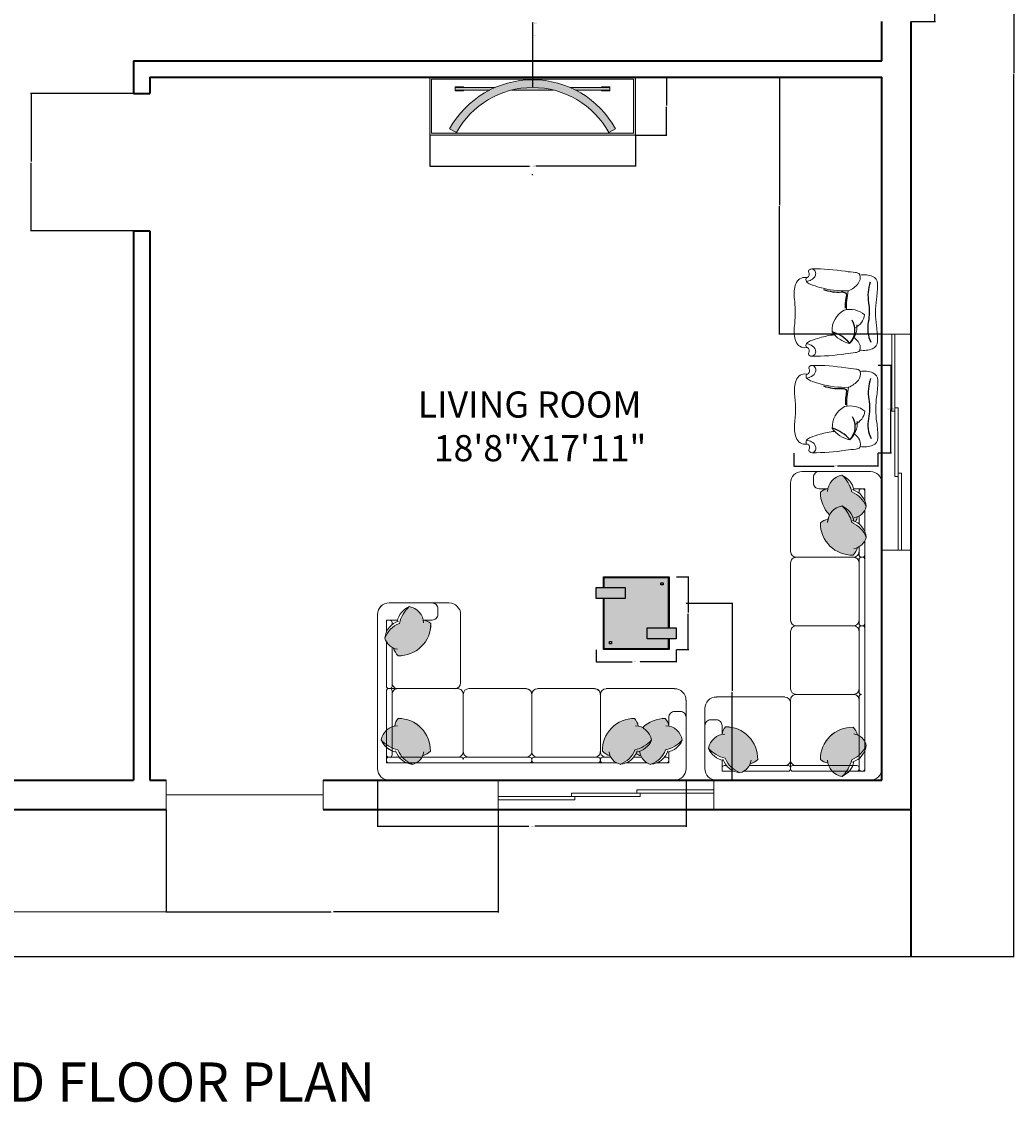
# Model space of a CAD drawing. Units: inches. Extents: x 1569 to 2779, y 1228 to 1844.
# Tile 2 of 6: x 1869 to 2173, y 1228 to 1559. Entities that reach past the tile are written whole.
import ezdxf

# ---------------------------------------------------------------- set-up
doc = ezdxf.new("R2010")
doc.units = ezdxf.units.IN
for name, color, linetype, lineweight in [('A-ANNO-DIMS', 2, 'Continuous', 18), ('A-ANNO-TEXT', 7, 'Continuous', 25), ('A-AREA-IDEN', 7, 'Continuous', 18), ('A-DOOR', 3, 'Continuous', 20), ('A-FLOR-EDGE', 7, 'Continuous', 25), ('A-FURN', 8, 'Continuous', 13), ('A-GLAZ', 5, 'Continuous', 18), ('A-WALL', 7, 'Continuous', 35), ('aparador', 36, 'Continuous', 9), ('moveis', 254, 'Continuous', 5)]:
    doc.layers.add(name, color=color, linetype=linetype, lineweight=lineweight)
doc.layers.add('IFF-FURN-DETAIL', color=250, linetype='Continuous')
doc.layers.add('MOBIL', color=7, linetype='Continuous')
doc.styles.get("Standard").update_dxf_attribs({"font": 'arial.ttf'})
doc.dimstyles.get("Standard").update_dxf_attribs({"dimtxt": 0.18, "dimasz": 0.18, "dimexe": 0.18, "dimexo": 0.0625, "dimgap": 0.09, "dimtad": 0, "dimtih": 1, "dimtoh": 1, "dimdec": 4, "dimzin": 0, "dimdsep": 46, "dimtxsty": 'Standard', "dimcen": 0.09, "dimadec": 0, "dimazin": 0, "dimtfac": 1, "dimtdec": 4, "dimtofl": 0, "dimtmove": 0, "dimatfit": 3, "dimfxl": 1, "dimtolj": 1, "dimtzin": 0, "dimarcsym": 0})

# ---------------------------------------------------------------- blocks, each defined once
blk = doc.blocks.new('Aparador ORGANICA Formatto')
at = {"layer": 'aparador', "ltscale": 0.3}
h = blk.add_hatch(color=256, dxfattribs=at)
h.dxf.hatch_style = 1
h.set_gradient(color1=(118, 213, 123), color2=(52, 168, 57), one_color=1, tint=0.43, name='INVCURVED')
h.paths.add_polyline_path([(0.8, 0.45), (-0.8, 0.45), (-0.8, 0), (0.8, 0)])
h.paths.add_polyline_path([(0.785, 0.435), (0.785, 0.015), (-0.785, 0.015), (-0.785, 0.435)], flags=16)
h.paths.add_polyline_path([(0.2911, 0.3699), (0.5365, 0.3699), (0.5365, 0.3757), (0.6011, 0.3757), (0.6011, 0.3699), (0.6011, 0.3499), (0.6011, 0.3441), (0.5365, 0.3441), (0.5365, 0.3499), (0.3338, 0.3499, -0.150336), (0.6449, 0.0488), (0.5923, 0.0199, 0.208852), (0.1632, 0.3499), (-0.1632, 0.3499, 0.208852), (-0.5923, 0.0199), (-0.6449, 0.0488, -0.150336), (-0.3338, 0.3499), (-0.5365, 0.3499), (-0.5365, 0.3441), (-0.6011, 0.3441), (-0.6011, 0.3499), (-0.6011, 0.3699), (-0.6011, 0.3757), (-0.5365, 0.3757), (-0.5365, 0.3699), (-0.2911, 0.3699, -0.206106)], flags=0)
h = blk.add_hatch(color=256, dxfattribs=at)
h.dxf.hatch_style = 1
h.set_gradient(color1=(135, 92, 69), color2=(0, 0, 0), one_color=1, name='INVCURVED')
h.paths.add_polyline_path([(-0.6449, 0.0488), (-0.5923, 0.0199, -0.590888), (0.5923, 0.0199), (0.6449, 0.0488, 0.590888)])
h = blk.add_hatch(color=256, dxfattribs=at)
h.dxf.hatch_style = 1
h.set_gradient(color1=(178, 189, 189), one_color=1, tint=1, name='CYLINDER')
h.paths.add_polyline_path([(-0.5365, 0.3757), (-0.6011, 0.3757), (-0.6011, 0.3699), (-0.5365, 0.3699)])
h.paths.add_polyline_path([(-0.5365, 0.3499), (-0.6011, 0.3499), (-0.6011, 0.3441), (-0.5365, 0.3441)])
h = blk.add_hatch(color=256, dxfattribs=at)
h.dxf.hatch_style = 1
h.set_gradient(color1=(118, 213, 123), color2=(31, 101, 35), one_color=1, tint=0.26, name='INVCURVED')
h.paths.add_polyline_path([(-0.2911, 0.3699), (-0.6011, 0.3699), (-0.6011, 0.3499), (-0.3338, 0.3499, -0.015999)])
h = blk.add_hatch(color=256, dxfattribs=at)
h.dxf.hatch_style = 1
h.set_gradient(color1=(118, 213, 123), color2=(31, 101, 35), one_color=1, tint=0.26, name='INVCURVED')
h.paths.add_polyline_path([(-0.1632, 0.3499), (0.1632, 0.3499, 0.122516)])
h = blk.add_hatch(color=256, dxfattribs=at)
h.dxf.hatch_style = 1
h.set_gradient(color1=(118, 213, 123), color2=(31, 101, 35), one_color=1, tint=0.26, name='INVCURVED')
h.paths.add_polyline_path([(0.6011, 0.3699), (0.2911, 0.3699, -0.015999), (0.3338, 0.3499), (0.6011, 0.3499)])
h = blk.add_hatch(color=256, dxfattribs=at)
h.dxf.hatch_style = 1
h.set_gradient(color1=(178, 189, 189), one_color=1, tint=1, name='CYLINDER')
h.paths.add_polyline_path([(0.6011, 0.3757), (0.5365, 0.3757), (0.5365, 0.3699), (0.6011, 0.3699)])
h.paths.add_polyline_path([(0.6011, 0.3499), (0.5365, 0.3499), (0.5365, 0.3441), (0.6011, 0.3441)])
for p, q in [((-0.5923, 0.0199), (-0.6449, 0.0488)), ((0.5923, 0.0199), (0.6449, 0.0488))]:
    blk.add_line(p, q, dxfattribs=at)
for points in [[(-0.6011, 0.3699), (-0.6011, 0.3757), (-0.5365, 0.3757), (-0.5365, 0.3699)], [(-0.5365, 0.3499), (-0.5365, 0.3441), (-0.6011, 0.3441), (-0.6011, 0.3499)], [(0.6011, 0.3699), (0.6011, 0.3757), (0.5365, 0.3757), (0.5365, 0.3699)], [(0.5365, 0.3499), (0.5365, 0.3441), (0.6011, 0.3441), (0.6011, 0.3499)]]:
    blk.add_lwpolyline(points, dxfattribs=at)
for radius in [0.7362, 0.6762]:
    blk.add_arc((0, -0.3063), radius, 28.84335, 151.15665, dxfattribs=at)
at = {"layer": 'moveis', "ltscale": 0.3}
for p, q in [((-0.6011, 0.3699), (-0.6011, 0.3499)), ((-0.2911, 0.3699), (-0.6011, 0.3699)), ((-0.6011, 0.3499), (-0.3338, 0.3499)), ((-0.1632, 0.3499), (0.1632, 0.3499)), ((0.2911, 0.3699), (0.6011, 0.3699)), ((0.6011, 0.3499), (0.3338, 0.3499)), ((0.6011, 0.3699), (0.6011, 0.3499))]:
    blk.add_line(p, q, dxfattribs=at)
for points in [[(-0.8, 0), (0.8, 0), (0.8, 0.45), (-0.8, 0.45)], [(-0.785, 0.015), (0.785, 0.015), (0.785, 0.435), (-0.785, 0.435)]]:
    blk.add_lwpolyline(points, close=True, dxfattribs=at)
blk = doc.blocks.new('SOFA 1')
at = {"transparency": 33554687}
h = blk.add_hatch(color=256, dxfattribs=at)
h.dxf.hatch_style = 1
h.paths.add_polyline_path([(3769.65, 1307.6, 0.084911), (3767.15, 1309.12, 0.046133), (3766.46, 1311.13), (3759.18, 1311.13, 0.039409), (3758.92, 1310.24, 0.165523), (3756.31, 1309.02, 0.42585), (3767.59, 1297.95, 0.121928), (3769.15, 1300.58, 0.027403), (3769.65, 1300.83)])
h.paths.add_polyline_path([(3765.34, 1313.08), (3760.4, 1313.08, 0.097704), (3759.18, 1311.13), (3766.46, 1311.13, 0.04873)])
h.paths.add_polyline_path([(3763.76, 1314.88, 0.16488), (3760.4, 1313.08), (3765.34, 1313.08, 0.051917)])
h.paths.add_polyline_path([(3771.6, 1305.17, 0.090388), (3769.65, 1307.6), (3769.65, 1300.83, 0.136035), (3771.6, 1302.77)])
h = blk.add_hatch(color=256, dxfattribs=at)
h.dxf.hatch_style = 1
h.paths.add_polyline_path([(3723.52, 1308.63, 0.147724), (3717.76, 1305.24, 0.310469), (3722.42, 1300.4), (3722.42, 1300.25, 0.156703), (3723.62, 1297.8, 0.425821), (3734.69, 1309.08, 0.121928), (3732.05, 1310.63, 0.233216), (3728.6, 1313.59, 0.213835)])
h = blk.add_hatch(color=256, dxfattribs=at)
h.dxf.hatch_style = 1
h.paths.add_polyline_path([(3769.16, 1235.96, 0.122267), (3767.6, 1238.61, 0.425972), (3756.32, 1227.54, 0.165563), (3758.93, 1226.32, 0.309481), (3763.76, 1221.69, 0.002677), (3763.83, 1221.72, 0.146094), (3767.16, 1227.43, 0.212433), (3772.1, 1232.48, 0.235342)])
h = blk.add_hatch(color=256, dxfattribs=at)
h.dxf.hatch_style = 1
h.paths.add_polyline_path([(3769.16, 1225.36, 0.122267), (3767.6, 1228.01, 0.425972), (3756.32, 1216.94, 0.165563), (3758.93, 1215.72, 0.309481), (3763.76, 1211.09, 0.002677), (3763.83, 1211.12, 0.146094), (3767.16, 1216.83, 0.212433), (3772.1, 1221.88, 0.235342)])
for p, q in [((3720.45, 1316.13), (3773.58, 1316.13)), ((3777.51, 1312.19), (3777.51, 1213.72))]:
    blk.add_line(p, q, dxfattribs=at)
for points in [[(3763.76, 1314.88, -0.147724), (3767.15, 1309.12, -0.213355), (3772.1, 1304.05, 0.213355), (3767.15, 1309.12, 0.147724), (3763.76, 1314.88, -0.249545), (3767.86, 1309.77, 0.249545), (3763.77, 1314.89, 0.356779), (3758.8, 1309.23, -0.356779), (3763.76, 1314.88)], [(3717.76, 1305.24, -0.147724), (3723.52, 1308.63, -0.213355), (3728.59, 1313.59, 0.213355), (3723.52, 1308.63, 0.147724), (3717.76, 1305.24, -0.249545), (3722.86, 1309.34, 0.249545), (3717.75, 1305.25, 0.356779), (3723.4, 1300.28, -0.356779), (3717.76, 1305.24)], [(3728.58, 1313.6, -0.306333), (3732.42, 1309.31, 0.306333), (3728.58, 1313.6, 0.306674), (3722.72, 1308.89, -0.306674), (3728.58, 1313.6)], [(3734.69, 1309.08, -0.425972), (3723.62, 1297.8, -0.165552), (3722.4, 1300.4, 0.165552), (3723.62, 1297.79, 0.425972), (3734.69, 1309.07, 0.121514), (3732.07, 1310.63, -0.121514), (3734.69, 1309.08)], [(3767.6, 1297.95, -0.425972), (3756.31, 1309.01, -0.165552), (3758.92, 1310.24, 0.165552), (3756.31, 1309.02, 0.425972), (3767.59, 1297.95, 0.121514), (3769.14, 1300.57, -0.121514), (3767.6, 1297.95)], [(3772.11, 1304.06, -0.306333), (3767.83, 1300.22, 0.306333), (3772.11, 1304.06, 0.306674), (3767.4, 1309.91, -0.306674), (3772.11, 1304.06)], [(3770.44, 1286.63, -0.414214), (3769.66, 1287.4, 0.414214), (3770.44, 1286.63, 0.414214), (3769.66, 1285.83, -0.414214), (3770.44, 1286.63)], [(3748.01, 1262.99, -0.414214), (3746.05, 1264.95, 0.414214), (3748.01, 1262.97, 0.414213), (3746.05, 1261.01, -0.414213), (3748.01, 1262.99)], [(3770.44, 1262.99, -0.414214), (3769.66, 1263.77, 0.414214), (3770.44, 1262.99, 0.414214), (3769.66, 1262.19, -0.414214), (3770.44, 1262.99)], [(3770.83, 1262.97, -0.414214), (3771.61, 1262.19, 0.414214), (3770.83, 1262.99, 0.414214), (3771.61, 1263.77, -0.414214), (3770.83, 1262.97)], [(3748.01, 1239.35, -0.414214), (3746.05, 1241.31, 0.414214), (3748.01, 1239.33, 0.414213), (3746.05, 1237.37, -0.414213), (3748.01, 1239.35)], [(3767.7, 1239.33, -0.414214), (3769.66, 1237.37, 0.414214), (3767.7, 1239.35, 0.414214), (3769.66, 1241.31, -0.414214), (3767.7, 1239.33)], [(3756.32, 1227.54, -0.425972), (3767.6, 1238.61, -0.121514), (3769.16, 1235.98, 0.121514), (3767.6, 1238.61, 0.425972), (3756.32, 1227.54, 0.165552), (3758.93, 1226.32, -0.165552), (3756.32, 1227.54)], [(3770.44, 1239.35, -0.414214), (3769.66, 1240.13, 0.414214), (3770.44, 1239.33, 0.414214), (3769.66, 1238.55, -0.414214), (3770.44, 1239.35)], [(3770.83, 1239.33, -0.414214), (3771.61, 1238.55, 0.414214), (3770.83, 1239.35, 0.414214), (3771.61, 1240.13, -0.414214), (3770.83, 1239.33)], [(3772.1, 1232.5, -0.306674), (3767.41, 1226.64, 0.306674), (3772.1, 1232.5, 0.306333), (3767.84, 1236.34, -0.306333), (3772.1, 1232.5)], [(3763.78, 1221.67, 0.249545), (3767.87, 1226.78, -0.249545), (3763.76, 1221.69, -0.356779), (3758.81, 1227.32, 0.356779), (3763.77, 1221.68, 0.147724), (3767.16, 1227.43, 0.213355), (3772.11, 1232.51, -0.213355), (3767.16, 1227.43, -0.147724), (3763.78, 1221.67)], [(3756.32, 1216.94, -0.200233), (3759.49, 1224.76, 0.200233), (3756.32, 1216.94, 0.165552), (3758.93, 1215.72, -0.165552), (3756.32, 1216.94)], [(3772.1, 1221.9, -0.306674), (3767.41, 1216.04, 0.306674), (3772.1, 1221.9, -0.213355), (3767.16, 1216.83, -0.147724), (3763.77, 1211.08, 0.147724), (3767.15, 1216.83, 0.213355), (3772.1, 1221.9)], [(3763.76, 1211.09, -0.356779), (3758.81, 1216.72, 0.356779), (3763.76, 1211.09, 0.249545), (3767.87, 1216.18, -0.249545), (3763.76, 1211.09)]]:
    blk.add_lwpolyline(points, format="xyb", dxfattribs=at)
for points in [[(3716.51, 1312.2), (3716.51, 1291.44)], [(3722.42, 1313.08), (3722.42, 1309.23), (3722.42, 1313.08), (3726.57, 1313.08)], [(3723.21, 1311.13), (3723.93, 1311.13)], [(3729.85, 1313.08), (3745.25, 1313.08)], [(3731.82, 1311.13), (3745.25, 1311.13)], [(3746.01, 1312.3), (3746.01, 1288.55)], [(3746.01, 1310.97), (3746.01, 1311.36)], [(3768.11, 1313.08), (3746.78, 1313.08)], [(3768.87, 1311.13), (3746.78, 1311.13)], [(3771.6, 1313.08), (3767.75, 1313.08), (3771.6, 1313.08), (3771.6, 1308.93)], [(3769.66, 1287.39), (3769.65, 1312.3)], [(3771.6, 1313.08), (3771.61, 1233.74)], [(3746.01, 1288.54), (3746.01, 1308.23)], [(3769.65, 1309.43), (3769.65, 1308.71)], [(3722.42, 1300.39), (3722.42, 1297.33)], [(3720.45, 1295.38), (3718.48, 1295.38)], [(3720.45, 1287.5), (3744.09, 1287.5)], [(3747.99, 1286.6), (3767.69, 1286.6)], [(3769.66, 1263.75), (3769.66, 1285.81)], [(3746.02, 1284.63), (3746.02, 1264.94)], [(3769.66, 1277.18), (3769.66, 1263.75)], [(3747.99, 1262.97), (3767.69, 1262.97)], [(3770.43, 1262.97), (3770.82, 1262.97)], [(3746.02, 1260.99), (3746.02, 1241.3)], [(3769.66, 1240.12), (3769.66, 1262.18)], [(3746.02, 1237.36), (3746.02, 1213.74)], [(3747.99, 1239.33), (3767.69, 1239.33)], [(3769.66, 1235.71), (3769.66, 1238.54)], [(3770.43, 1239.33), (3770.82, 1239.33)], [(3771.61, 1223.14), (3771.61, 1230.47)], [(3769.66, 1225.11), (3769.66, 1227.82)], [(3767.76, 1215.72), (3771.61, 1215.72), (3771.61, 1219.84), (3771.61, 1215.72)], [(3755.86, 1215.72), (3758.92, 1215.72)], [(3769.66, 1216.5), (3769.66, 1217.22)], [(3753.91, 1211.77), (3753.91, 1213.74)], [(3749.97, 1209.8), (3773.58, 1209.8)]]:
    blk.add_lwpolyline(points, close=True, dxfattribs=at)
for points in [[(3722.42, 1311.91, 0.414214), (3723.2, 1311.13, -0.414214)], [(3770.43, 1313.08, 0.414214), (3769.65, 1312.3, -0.414214)], [(3771.6, 1312.3, 0.414214), (3770.82, 1313.08, -0.414214)], [(3716.51, 1297.34, 0.414214), (3718.47, 1295.38, -0.414214)], [(3720.44, 1295.38, 0.414214), (3722.4, 1297.34, -0.414214)], [(3716.51, 1291.45, 0.414212), (3720.44, 1287.52, -0.414212)], [(3746.03, 1288.56, 0.414214), (3747.99, 1286.6, 0.414213), (3746.03, 1284.64, -0.414213), (3747.99, 1286.6, -0.414214)], [(3769.66, 1284.64, 0.414214), (3767.7, 1286.6, 0.414214), (3769.66, 1288.56, -0.414214), (3767.7, 1286.6, -0.414214)], [(3769.66, 1261.01, 0.414214), (3767.7, 1262.97, 0.414214), (3769.66, 1264.93, -0.414214), (3767.7, 1262.97, -0.414214)], [(3772.13, 1221.9, 0.306333), (3767.84, 1225.74, -0.306333)], [(3769.16, 1225.36, 0.071861), (3768.39, 1227.01, -0.071861)], [(3755.87, 1215.72, 0.414214), (3753.91, 1213.76, -0.414214)], [(3769.66, 1216.52, 0.414214), (3770.44, 1215.74, -0.414214)], [(3770.83, 1215.74, 0.414214), (3771.61, 1216.52, -0.414214)], [(3746.05, 1213.76, 0.414212), (3749.98, 1209.82, -0.414212)], [(3755.87, 1209.8, -0.414214), (3753.91, 1211.76, 0.414214)]]:
    blk.add_lwpolyline(points, format="xyb", close=True, dxfattribs=at)
for centre, radius, start, end in [((3720.44, 1312.2), 3.93, 90.0002, 179.9998), ((3720.44, 1312.19), 3.94, 89.9158, 179.9154), ((3773.58, 1312.2), 3.93, 0.0002, 89.9998), ((3773.57, 1312.19), 3.94, 359.9158, 89.9154), ((3744.09, 1309.21), 1.92, 358.766, 90.5111), ((3745.22, 1312.29), 0.789, 0.8425, 90.8425), ((3745.24, 1311.91), 0.777, 270, 0), ((3745.24, 1311.91), 0.777, 270, 0), ((3746.8, 1312.29), 0.789, 89.1575, 179.1575), ((3746.79, 1311.91), 0.777, 180, 270), ((3746.79, 1311.91), 0.777, 180, 270), ((3747.93, 1309.21), 1.92, 89.4889, 181.234), ((3768.87, 1312.3), 0.777, 360, 90), ((3768.87, 1311.91), 0.777, 270, 0), ((3744.08, 1289.48), 1.96, 270, 360), ((3744.08, 1289.48), 1.96, 270, 360), ((3773.58, 1213.73), 3.93, 270.0002, 359.9998), ((3773.59, 1213.73), 3.93, 269.9156, 359.9152)]:
    blk.add_arc(centre, radius, start, end, dxfattribs=at)
blk = doc.blocks.new('Mesa de centro Cantria feeling')
at = {"layer": 'MOBIL', "ltscale": 0.2}
h = blk.add_hatch(color=256, dxfattribs=at)
h.set_gradient(color1=(74, 55, 38), color2=(104, 77, 54), one_color=1, tint=0.31, name='CYLINDER')
h.paths.add_polyline_path([(-0.85, -0.3), (-0.7, -0.3), (-0.7, 0.1), (-0.85, 0.1)])
h = blk.add_hatch(color=256, dxfattribs=at)
h.set_gradient(color1=(221, 221, 223), one_color=1, tint=1)
h.paths.add_polyline_path([(-0.15, -0.6), (-0.15, -0.89), (-0.01, -0.89), (-0.01, -0.01), (-0.7, -0.01), (-0.7, -0.3), (-0.85, -0.3), (-0.85, -0.01), (-0.99, -0.01), (-0.99, -0.89), (-0.3, -0.89), (-0.3, -0.6)])
h.paths.add_polyline_path([(-0.112, -0.112), (-0.112, -0.082), (-0.082, -0.082), (-0.082, -0.112)], flags=16)
h.paths.add_polyline_path([(-0.888, -0.788), (-0.888, -0.818), (-0.918, -0.818), (-0.918, -0.788)], flags=16)
h = blk.add_hatch(color=256, dxfattribs=at)
h.set_gradient(color1=(74, 55, 38), color2=(104, 77, 54), one_color=1, tint=0.31, name='CYLINDER')
h.paths.add_polyline_path([(-0.15, -0.6), (-0.3, -0.6), (-0.3, -1), (-0.15, -1)])
for points in [[(-0.85, 0), (-1, 0), (-1, -0.9), (-0.3, -0.9)], [(-0.15, -0.9), (0, -0.9), (0, 0), (-0.7, 0)], [(-0.85, -0.01), (-0.99, -0.01), (-0.99, -0.89), (-0.3, -0.89)], [(-0.15, -0.89), (-0.01, -0.89), (-0.01, -0.01), (-0.7, -0.01)]]:
    blk.add_lwpolyline(points, dxfattribs=at)
for points in [[(-0.85, -0.3), (-0.7, -0.3), (-0.7, 0.1), (-0.85, 0.1)], [(-0.082, -0.082), (-0.112, -0.082), (-0.112, -0.112), (-0.082, -0.112)], [(-0.15, -0.6), (-0.3, -0.6), (-0.3, -1), (-0.15, -1)], [(-0.918, -0.818), (-0.888, -0.818), (-0.888, -0.788), (-0.918, -0.788)]]:
    blk.add_lwpolyline(points, close=True, dxfattribs=at)
blk = doc.blocks.new('PILLOW-1')
at = {"color": 0}
blk.add_lwpolyline([(198, -165, -0.232884), (126, -346, -0.184752), (-44, -234, -0.286563), (75, -22, -0.237978), (273, -68, -0.243587), (179, -195, 4.263709)], format="xyb", dxfattribs=at)
at = {"layer": 'IFF-FURN-DETAIL'}
blk.add_lwpolyline([(148, -118, -0.343333), (126, -342, 0.126408), (-40, -233, -5.969376)], format="xyb", dxfattribs=at)
blk = doc.blocks.new('CLNG90')
for points in [[(689, 370, 0.157831), (677, 385, 0.121013), (646, 395, -0.017334), (547, 407, 0.041496), (215, 431, 0.153531), (191, 423, 0.382906), (185, 395, -0.284047), (184, 361, 0.011997), (177, 351, -0.370479), (160, 345, 0.380647), (56, 282, 0.117468), (41, 146, -0.027775), (50, 0, -8.773898)], [(160, 345, 0.22481), (160, 306, 0.055398), (209, 322, 0.180116), (249, 368, 0.194833), (248, 405, 0.242377), (215, 431, 1.52074)], [(160, 345, 0.22481), (160, 306, 0.055398), (209, 322, 0.180116), (249, 368, 0.194833), (248, 405, 0.242377), (215, 431, 1.52074)], [(689, 370, -0.235486), (671, 286, -0.134038), (574, 215, -0.079303), (293, 248, -0.027048), (199, 280, -0.106276), (160, 306, -1.699)], [(689, 370, -0.235486), (671, 286, -0.134038), (574, 215, -0.079303), (293, 248, -0.027048), (199, 280, -0.106276), (160, 306, -1.699)], [(689, 370, -0.146607), (814, 357, -0.305296), (862, 286, -0.042137), (852, 131, 0.040285), (843, 0, 3.952121)], [(574, 215, 0.061244), (556, 29, 3.376255)], [(574, 215, 0.061244), (556, 29, 3.376255)], [(689, -370, -0.157831), (677, -385, -0.121013), (646, -395, 0.017334), (547, -407, -0.041496), (215, -431, -0.153531), (191, -423, -0.382906), (185, -395, 0.284047), (184, -361, -0.011997), (177, -351, 0.370479), (160, -345, -0.380647), (56, -282, -0.117468), (41, -146, 0.027775), (50, 0, 8.773898)], [(689, -370, 0.146607), (814, -357, 0.305296), (862, -286, 0.042137), (852, -131, -0.040285), (843, 0, -3.952121)], [(160, -345, -0.22481), (160, -306, -0.055398), (209, -322, -0.180116), (249, -368, -0.194833), (248, -405, -0.242377), (215, -431, -1.52074)], [(160, -345, -0.22481), (160, -306, -0.055398), (209, -322, -0.180116), (249, -368, -0.194833), (248, -405, -0.242377), (215, -431, -1.52074)], [(437, -220, 0.041086), (293, -248, 0.027048), (199, -280, 0.106276), (160, -306, 1.699)], [(437, -220, 0.041086), (293, -248, 0.027048), (199, -280, 0.106276), (160, -306, 1.699)], [(689, -370, 0.235486), (671, -286, 0.060693), (632, -247, 0.001296)], [(689, -370, 0.235486), (671, -286, 0.060693), (632, -247, 0.001296)]]:
    blk.add_lwpolyline(points, format="xyb")
at = {"layer": 'IFF-FURN-DETAIL'}
for points in [[(328, 228, 0.109125), (508, 203, -0.16587), (546, 194, -0.314359), (555, 172, 0.072017), (544, 42, 4.351186)], [(328, 228, 0.109125), (508, 203, -0.16587), (546, 194, -0.314359), (555, 172, 0.072017), (544, 42, 4.351186)], [(791, 301, 0.124986), (774, 96, -0.091334), (771, -95, 0.164688), (797, -292, 1.068868)], [(791, 301, 0.124986), (774, 96, -0.091334), (771, -95, 0.164688), (797, -292, 1.068868)]]:
    blk.add_lwpolyline(points, format="xyb", dxfattribs=at)
at = {"xscale": 1.016, "yscale": 1.016, "zscale": 1.016}
blk.add_blockref('PILLOW-1', (458, 47), dxfattribs=at)
blk.add_blockref('PILLOW-1', (458, 47), dxfattribs=at)
blk = doc.blocks.new('WIN-66IN')
for p, q in [((0, 0), (0, 9)), ((66, 0), (66, 9)), ((0, 4), (43.5, 4)), ((22.5, 5), (66, 5)), ((22.5, 4), (22.5, 5)), ((23.5, 3), (23.5, 4)), ((42.5, 6), (66, 6)), ((42.5, 5), (42.5, 6)), ((43.5, 4), (43.5, 5)), ((0, 3), (23.5, 3))]:
    blk.add_line(p, q)
blk = doc.blocks.new('DOOR-48IN')
for p, q in [((0, 0), (0, 9)), ((48, 0), (48, 9)), ((48, 4.5), (0, 4.5))]:
    blk.add_line(p, q)
blk = doc.blocks.new('*D17')
at = {"layer": 'A-ANNO-DIMS', "color": 0, "lineweight": -2, "transparency": 16777216}
for p, q in [((2141.09, 1606.88), (2148.41, 1606.88)), ((2148.23, 1606.7), (2148.23, 1583.06)), ((2148.23, 1559.06), (2148.23, 1582.7)), ((2141.09, 1558.88), (2148.41, 1558.88))]:
    blk.add_line(p, q, dxfattribs=at)
at = {"layer": 'A-ANNO-DIMS', "color": 0, "transparency": 16777216}
for points in [[(2148.2, 1606.7), (2148.26, 1606.7), (2148.23, 1606.88)], [(2148.2, 1559.06), (2148.26, 1559.06), (2148.23, 1558.88)]]:
    blk.add_solid(points, dxfattribs=at)
at = {"layer": 'Defpoints', "color": 0, "transparency": 16777216}
for p in [(2141.03, 1606.88), (2148.23, 1606.88), (2141.03, 1558.88)]:
    blk.add_point(p, dxfattribs=at)
at = {"layer": 'A-ANNO-DIMS', "color": 0, "transparency": 16777216, "insert": (2148.23, 1582.88), "char_height": 0.18, "attachment_point": 5}
blk.add_mtext('\\A1;ENTRY DOOR 48 TYP.', dxfattribs=at)
blk = doc.blocks.new('*D39')
at = {"layer": 'A-ANNO-DIMS', "color": 0, "lineweight": -2, "transparency": 16777216}
for p, q in [((1977.71, 1326.83), (1977.71, 1312.55)), ((2072.1, 1326.83), (2072.1, 1312.55)), ((1977.89, 1312.73), (2024, 1312.73)), ((2071.92, 1312.73), (2025.81, 1312.73))]:
    blk.add_line(p, q, dxfattribs=at)
at = {"layer": 'A-ANNO-DIMS', "color": 0, "transparency": 16777216}
for points in [[(1977.89, 1312.76), (1977.89, 1312.7), (1977.71, 1312.73)], [(2071.92, 1312.76), (2071.92, 1312.7), (2072.1, 1312.73)]]:
    blk.add_solid(points, dxfattribs=at)
at = {"layer": 'Defpoints', "color": 0, "transparency": 16777216}
for p in [(1977.71, 1326.89), (2072.1, 1326.89), (1977.71, 1312.73)]:
    blk.add_point(p, dxfattribs=at)
at = {"layer": 'A-ANNO-DIMS', "color": 0, "transparency": 16777216, "insert": (2024.9, 1312.73), "char_height": 0.18, "attachment_point": 5}
blk.add_mtext('\\A1;SOFA 94 TYP.', dxfattribs=at)
blk = doc.blocks.new('*D40')
at = {"layer": 'A-ANNO-DIMS', "color": 0, "lineweight": -2, "transparency": 16777216}
for p, q in [((2072.16, 1381.04), (2086.44, 1381.04)), ((2086.26, 1380.86), (2086.26, 1354.15)), ((2086.26, 1327.07), (2086.26, 1353.79)), ((2072.16, 1326.89), (2086.44, 1326.89))]:
    blk.add_line(p, q, dxfattribs=at)
at = {"layer": 'A-ANNO-DIMS', "color": 0, "transparency": 16777216}
for points in [[(2086.23, 1380.86), (2086.29, 1380.86), (2086.26, 1381.04)], [(2086.23, 1327.07), (2086.29, 1327.07), (2086.26, 1326.89)]]:
    blk.add_solid(points, dxfattribs=at)
at = {"layer": 'Defpoints', "color": 0, "transparency": 16777216}
for p in [(2072.1, 1381.04), (2072.1, 1326.89), (2086.26, 1326.89)]:
    blk.add_point(p, dxfattribs=at)
at = {"layer": 'A-ANNO-DIMS', "color": 0, "transparency": 16777216, "insert": (2086.26, 1353.97), "char_height": 0.18, "attachment_point": 5}
blk.add_mtext('\\A1;54 TYP.', dxfattribs=at)
blk = doc.blocks.new('*D41')
at = {"layer": 'A-ANNO-DIMS', "color": 0, "lineweight": -2, "transparency": 16777216}
for p, q in [((2130.86, 1453.77), (2135, 1453.77)), ((2134.82, 1453.59), (2134.82, 1440.55)), ((2134.82, 1427.14), (2134.82, 1440.18)), ((2130.86, 1426.96), (2135, 1426.96))]:
    blk.add_line(p, q, dxfattribs=at)
at = {"layer": 'A-ANNO-DIMS', "color": 0, "transparency": 16777216}
for points in [[(2134.79, 1453.59), (2134.85, 1453.59), (2134.82, 1453.77)], [(2134.79, 1427.14), (2134.85, 1427.14), (2134.82, 1426.96)]]:
    blk.add_solid(points, dxfattribs=at)
at = {"layer": 'Defpoints', "color": 0, "transparency": 16777216}
for p in [(2130.79, 1453.77), (2134.82, 1453.77), (2130.79, 1426.96)]:
    blk.add_point(p, dxfattribs=at)
at = {"layer": 'A-ANNO-DIMS', "color": 0, "transparency": 16777216, "insert": (2134.82, 1440.36), "char_height": 0.18, "attachment_point": 5}
blk.add_mtext('\\A1;ARMCHAIR 27 TYP.', dxfattribs=at)
blk = doc.blocks.new('*D42')
at = {"layer": 'A-ANNO-DIMS', "color": 0, "lineweight": -2, "transparency": 16777216}
for p, q in [((2105.13, 1426.89), (2105.13, 1422.75)), ((2130.79, 1426.89), (2130.79, 1422.75)), ((2105.31, 1422.93), (2117.43, 1422.93)), ((2130.61, 1422.93), (2118.49, 1422.93))]:
    blk.add_line(p, q, dxfattribs=at)
at = {"layer": 'A-ANNO-DIMS', "color": 0, "transparency": 16777216}
for points in [[(2105.31, 1422.96), (2105.31, 1422.9), (2105.13, 1422.93)], [(2130.61, 1422.96), (2130.61, 1422.9), (2130.79, 1422.93)]]:
    blk.add_solid(points, dxfattribs=at)
at = {"layer": 'Defpoints', "color": 0, "transparency": 16777216}
for p in [(2105.13, 1426.96), (2130.79, 1426.96), (2130.79, 1422.93)]:
    blk.add_point(p, dxfattribs=at)
at = {"layer": 'A-ANNO-DIMS', "color": 0, "transparency": 16777216, "insert": (2117.96, 1422.93), "char_height": 0.18, "attachment_point": 5}
blk.add_mtext('\\A1;26 TYP.', dxfattribs=at)
blk = doc.blocks.new('*D43')
at = {"layer": 'A-ANNO-DIMS', "color": 0, "lineweight": -2, "transparency": 16777216}
for p, q in [((1993.65, 1524.1), (1993.65, 1514.53)), ((2056.65, 1524.1), (2056.65, 1514.53)), ((1993.83, 1514.71), (2024.16, 1514.71)), ((2056.47, 1514.71), (2026.14, 1514.71))]:
    blk.add_line(p, q, dxfattribs=at)
at = {"layer": 'A-ANNO-DIMS', "color": 0, "transparency": 16777216}
for points in [[(1993.83, 1514.74), (1993.83, 1514.68), (1993.65, 1514.71)], [(2056.47, 1514.74), (2056.47, 1514.68), (2056.65, 1514.71)]]:
    blk.add_solid(points, dxfattribs=at)
at = {"layer": 'Defpoints', "color": 0, "transparency": 16777216}
for p in [(1993.65, 1524.16), (2056.65, 1524.16), (2056.65, 1514.71)]:
    blk.add_point(p, dxfattribs=at)
at = {"layer": 'A-ANNO-DIMS', "color": 0, "transparency": 16777216, "insert": (2025.15, 1514.71), "char_height": 0.18, "attachment_point": 5}
blk.add_mtext('\\A1;SIDEBOARD 63', dxfattribs=at)
blk = doc.blocks.new('*D44')
at = {"layer": 'A-ANNO-DIMS', "color": 0, "lineweight": -2, "transparency": 16777216}
for p, q in [((2056.71, 1541.88), (2066.27, 1541.88)), ((2066.09, 1541.7), (2066.09, 1533.2)), ((2066.09, 1524.34), (2066.09, 1532.84)), ((2056.71, 1524.16), (2066.27, 1524.16))]:
    blk.add_line(p, q, dxfattribs=at)
at = {"layer": 'A-ANNO-DIMS', "color": 0, "transparency": 16777216}
for points in [[(2066.06, 1541.7), (2066.12, 1541.7), (2066.09, 1541.88)], [(2066.06, 1524.34), (2066.12, 1524.34), (2066.09, 1524.16)]]:
    blk.add_solid(points, dxfattribs=at)
at = {"layer": 'Defpoints', "color": 0, "transparency": 16777216}
for p in [(2056.65, 1541.88), (2066.09, 1541.88), (2056.65, 1524.16)]:
    blk.add_point(p, dxfattribs=at)
at = {"layer": 'A-ANNO-DIMS', "color": 0, "transparency": 16777216, "insert": (2066.09, 1533.02), "char_height": 0.18, "attachment_point": 5}
blk.add_mtext('\\A1;18', dxfattribs=at)
blk = doc.blocks.new('*D45')
at = {"layer": 'A-ANNO-DIMS', "color": 0, "lineweight": -2, "transparency": 16777216}
for p, q in [((2044.57, 1366.71), (2044.57, 1362.91)), ((2069.12, 1366.71), (2069.12, 1362.91)), ((2044.75, 1363.09), (2055.65, 1363.09)), ((2068.94, 1363.09), (2058.04, 1363.09))]:
    blk.add_line(p, q, dxfattribs=at)
at = {"layer": 'A-ANNO-DIMS', "color": 0, "transparency": 16777216}
for points in [[(2044.75, 1363.12), (2044.75, 1363.06), (2044.57, 1363.09)], [(2068.94, 1363.12), (2068.94, 1363.06), (2069.12, 1363.09)]]:
    blk.add_solid(points, dxfattribs=at)
at = {"layer": 'Defpoints', "color": 0, "transparency": 16777216}
for p in [(2044.57, 1366.77), (2069.12, 1366.77), (2044.57, 1363.09)]:
    blk.add_point(p, dxfattribs=at)
at = {"layer": 'A-ANNO-DIMS', "color": 0, "transparency": 16777216, "insert": (2056.85, 1363.09), "char_height": 0.18, "attachment_point": 5}
blk.add_mtext('\\A1;COFFEE TABLE 25', dxfattribs=at)
blk = doc.blocks.new('*D46')
at = {"layer": 'A-ANNO-DIMS', "color": 0, "lineweight": -2, "transparency": 16777216}
for p, q in [((2069.18, 1389.08), (2072.98, 1389.08)), ((2072.8, 1388.9), (2072.8, 1378.1)), ((2072.8, 1366.95), (2072.8, 1377.74)), ((2069.18, 1366.77), (2072.98, 1366.77))]:
    blk.add_line(p, q, dxfattribs=at)
at = {"layer": 'A-ANNO-DIMS', "color": 0, "transparency": 16777216}
for points in [[(2072.77, 1388.9), (2072.83, 1388.9), (2072.8, 1389.08)], [(2072.77, 1366.95), (2072.83, 1366.95), (2072.8, 1366.77)]]:
    blk.add_solid(points, dxfattribs=at)
at = {"layer": 'Defpoints', "color": 0, "transparency": 16777216}
for p in [(2069.12, 1389.08), (2069.12, 1366.77), (2072.8, 1366.77)]:
    blk.add_point(p, dxfattribs=at)
at = {"layer": 'A-ANNO-DIMS', "color": 0, "transparency": 16777216, "insert": (2072.8, 1377.92), "char_height": 0.18, "attachment_point": 5}
blk.add_mtext('\\A1;22', dxfattribs=at)
blk = doc.blocks.new('*D48')
at = {"layer": 'A-ANNO-DIMS', "color": 0, "lineweight": -2, "transparency": 16777216}
for p, q in [((2141.09, 1812.88), (2172.56, 1812.88)), ((2172.38, 1812.7), (2172.38, 1543.06)), ((2172.38, 1273.06), (2172.38, 1542.7)), ((2141.09, 1272.88), (2172.56, 1272.88))]:
    blk.add_line(p, q, dxfattribs=at)
at = {"layer": 'A-ANNO-DIMS', "color": 0, "transparency": 16777216}
for points in [[(2172.35, 1812.7), (2172.41, 1812.7), (2172.38, 1812.88)], [(2172.35, 1273.06), (2172.41, 1273.06), (2172.38, 1272.88)]]:
    blk.add_solid(points, dxfattribs=at)
at = {"layer": 'Defpoints', "color": 0, "transparency": 16777216}
for p in [(2141.03, 1812.88), (2172.38, 1812.88), (2141.03, 1272.88)]:
    blk.add_point(p, dxfattribs=at)
at = {"layer": 'A-ANNO-DIMS', "color": 0, "transparency": 16777216, "insert": (2172.38, 1542.88), "char_height": 0.18, "attachment_point": 5}
blk.add_mtext('\\A1;540', dxfattribs=at)
blk = doc.blocks.new('*D59')
at = {"layer": 'A-ANNO-DIMS', "color": 0, "lineweight": -2, "transparency": 16777216}
for p, q in [((1800.03, 1317.8), (1800.04, 1286.33)), ((1913.03, 1317.82), (1913.04, 1286.35)), ((1800.22, 1286.51), (1856.26, 1286.52)), ((1912.86, 1286.53), (1856.82, 1286.52))]:
    blk.add_line(p, q, dxfattribs=at)
at = {"layer": 'A-ANNO-DIMS', "color": 0, "transparency": 16777216}
for points in [[(1800.22, 1286.54), (1800.22, 1286.48), (1800.04, 1286.51)], [(1912.86, 1286.56), (1912.86, 1286.5), (1913.04, 1286.53)]]:
    blk.add_solid(points, dxfattribs=at)
at = {"layer": 'Defpoints', "color": 0, "transparency": 16777216}
for p in [(1800.03, 1317.86), (1913.03, 1317.88), (1800.04, 1286.51)]:
    blk.add_point(p, dxfattribs=at)
at = {"layer": 'A-ANNO-DIMS', "color": 0, "transparency": 16777216, "insert": (1856.54, 1286.52), "char_height": 0.18, "attachment_point": 5}
blk.add_mtext('\\A1;113', dxfattribs=at)
blk = doc.blocks.new('*D60')
at = {"layer": 'A-ANNO-DIMS', "color": 0, "lineweight": -2, "transparency": 16777216}
for p, q in [((1913.03, 1317.82), (1913.03, 1286.35)), ((2014.57, 1317.82), (2014.57, 1286.35)), ((1913.21, 1286.53), (1963.35, 1286.53)), ((2014.39, 1286.53), (1964.26, 1286.53))]:
    blk.add_line(p, q, dxfattribs=at)
at = {"layer": 'A-ANNO-DIMS', "color": 0, "transparency": 16777216}
for points in [[(1913.21, 1286.56), (1913.21, 1286.5), (1913.03, 1286.53)], [(2014.39, 1286.56), (2014.39, 1286.5), (2014.57, 1286.53)]]:
    blk.add_solid(points, dxfattribs=at)
at = {"layer": 'Defpoints', "color": 0, "transparency": 16777216}
for p in [(1913.03, 1317.88), (2014.57, 1317.88), (1913.03, 1286.53)]:
    blk.add_point(p, dxfattribs=at)
at = {"layer": 'A-ANNO-DIMS', "color": 0, "transparency": 16777216, "insert": (1963.8, 1286.53), "char_height": 0.18, "attachment_point": 5}
blk.add_mtext('\\A1;101.54', dxfattribs=at)
blk = doc.blocks.new('*D68')
at = {"layer": 'A-ANNO-DIMS', "color": 0, "lineweight": -2, "transparency": 16777216}
for p, q in [((2131.97, 1541.88), (2100.5, 1541.88)), ((2100.68, 1541.7), (2100.68, 1502.75)), ((2100.68, 1463.43), (2100.68, 1502.38)), ((2131.97, 1463.25), (2100.5, 1463.25))]:
    blk.add_line(p, q, dxfattribs=at)
at = {"layer": 'A-ANNO-DIMS', "color": 0, "transparency": 16777216}
for points in [[(2100.65, 1541.7), (2100.71, 1541.7), (2100.68, 1541.88)], [(2100.65, 1463.43), (2100.71, 1463.43), (2100.68, 1463.25)]]:
    blk.add_solid(points, dxfattribs=at)
at = {"layer": 'Defpoints', "color": 0, "transparency": 16777216}
for p in [(2100.68, 1541.88), (2132.03, 1541.88), (2132.03, 1463.25)]:
    blk.add_point(p, dxfattribs=at)
at = {"layer": 'A-ANNO-DIMS', "color": 0, "transparency": 16777216, "insert": (2100.68, 1502.56), "char_height": 0.18, "attachment_point": 5}
blk.add_mtext('\\A1;78.63', dxfattribs=at)
blk = doc.blocks.new('*D82')
at = {"layer": 'A-ANNO-DIMS', "color": 0, "lineweight": -2, "transparency": 16777216}
for p, q in [((1902.97, 1536.88), (1871.5, 1536.88)), ((1871.68, 1536.7), (1871.68, 1516.06)), ((1871.68, 1495.06), (1871.68, 1515.7)), ((1902.97, 1494.88), (1871.5, 1494.88))]:
    blk.add_line(p, q, dxfattribs=at)
at = {"layer": 'A-ANNO-DIMS', "color": 0, "transparency": 16777216}
for points in [[(1871.65, 1536.7), (1871.71, 1536.7), (1871.68, 1536.88)], [(1871.65, 1495.06), (1871.71, 1495.06), (1871.68, 1494.88)]]:
    blk.add_solid(points, dxfattribs=at)
at = {"layer": 'Defpoints', "color": 0, "transparency": 16777216}
for p in [(1871.68, 1536.88), (1903.03, 1536.88), (1903.03, 1494.88)]:
    blk.add_point(p, dxfattribs=at)
at = {"layer": 'A-ANNO-DIMS', "color": 0, "transparency": 16777216, "insert": (1871.68, 1515.88), "char_height": 0.18, "attachment_point": 5}
blk.add_mtext('\\A1;42', dxfattribs=at)
blk = doc.blocks.new('*D84')
at = {"layer": 'A-ANNO-DIMS', "color": 0, "lineweight": -2, "transparency": 16777216}
for p, q in [((2025.33, 1558.48), (2025.15, 1558.48)), ((2025.15, 1558.48), (2025.15, 1541.27)), ((2025.06, 1512.1), (2025.24, 1512.1)), ((2025.15, 1512.01), (2025.15, 1512.19))]:
    blk.add_line(p, q, dxfattribs=at)
at = {"layer": 'A-ANNO-DIMS', "color": 0, "transparency": 16777216}
blk.add_solid([(2025.12, 1541.27), (2025.18, 1541.27), (2025.15, 1541.09)], dxfattribs=at)
at = {"layer": 'Defpoints', "color": 0, "transparency": 16777216}
for p in [(2025.15, 1541.09), (2025.15, 1512.1)]:
    blk.add_point(p, dxfattribs=at)
at = {"layer": 'A-ANNO-DIMS', "color": 0, "transparency": 16777216, "insert": (2025.88, 1558.48), "char_height": 0.18, "attachment_point": 5}
blk.add_mtext('\\A1;R28.985', dxfattribs=at)
blk = doc.blocks.new('*D85')
at = {"layer": 'A-ANNO-DIMS', "color": 0, "lineweight": -2, "transparency": 16777216}
for p, q in [((2025.33, 1554.7), (2025.15, 1554.7)), ((2025.15, 1554.7), (2025.15, 1538.9)), ((2025.06, 1512.1), (2025.24, 1512.1)), ((2025.15, 1512.01), (2025.15, 1512.19))]:
    blk.add_line(p, q, dxfattribs=at)
at = {"layer": 'A-ANNO-DIMS', "color": 0, "transparency": 16777216}
blk.add_solid([(2025.12, 1538.9), (2025.18, 1538.9), (2025.15, 1538.72)], dxfattribs=at)
at = {"layer": 'Defpoints', "color": 0, "transparency": 16777216}
for p in [(2025.15, 1538.72), (2025.15, 1512.1)]:
    blk.add_point(p, dxfattribs=at)
at = {"layer": 'A-ANNO-DIMS', "color": 0, "transparency": 16777216, "insert": (2025.88, 1554.7), "char_height": 0.18, "attachment_point": 5}
blk.add_mtext('\\A1;R26.623', dxfattribs=at)

msp = doc.modelspace()

# ---------------------------------------------------------------- linework, layer by layer
at = {"layer": 'A-FLOR-EDGE'}
msp.add_line((1601.032, 1272.8785), (2141.032, 1272.8785), dxfattribs=at)
at = {"layer": 'A-WALL'}
for p, q in [((2132.032, 1546.8785), (2132.032, 1558.8785)), ((2141.032, 1272.8785), (2141.032, 1558.8785)), ((1903.032, 1546.8785), (1903.032, 1536.8785)), ((1903.032, 1546.8785), (2132.032, 1546.8785)), ((1908.032, 1541.8785), (1908.032, 1536.8785)), ((1908.032, 1541.8785), (2132.032, 1541.8785)), ((2132.032, 1326.8785), (2132.032, 1541.8785)), ((1903.032, 1536.8785), (1908.032, 1536.8785)), ((1903.032, 1494.8785), (1908.032, 1494.8785)), ((1903.032, 1494.8785), (1903.032, 1326.8785)), ((1908.032, 1494.8785), (1908.032, 1326.8785)), ((1763.032, 1326.8785), (1903.032, 1326.8785)), ((1908.032, 1326.8785), (1913.032, 1326.8785)), ((1961.032, 1326.8785), (2132.032, 1326.8785)), ((1601.032, 1317.8785), (1913.032, 1317.8785)), ((1961.032, 1317.8785), (2141.032, 1317.8785))]:
    msp.add_line(p, q, dxfattribs=at)

# ---------------------------------------------------------------- block references
at = {"layer": 'A-DOOR', "rotation": 180}
msp.add_blockref('DOOR-48IN', (1961.032, 1326.8785), dxfattribs=at)
at = {"layer": 'A-FURN'}
for name, p, xscale, yscale, zscale in [('Aparador ORGANICA Formatto', (2025.1497, 1524.1619), 39.3701, 39.3701, 39.3701), ('CLNG90', (2103.9595, 1469.8852), 0.031001591544, 0.031001591544, 0.031001591544), ('CLNG90', (2104.0458, 1440.3637), 0.031001591544, 0.031001591544, 0.031001591544)]:
    msp.add_blockref(name, p, dxfattribs=dict(at, xscale=xscale, yscale=yscale, zscale=zscale))
for name, p, xscale, yscale, zscale, rotation in [('SOFA 1', (-1221.0883, 2495.1463), -0.887653230693335, 0.887653230693335, 0.887653230693335, 180), ('Mesa de centro Cantria feeling', (2046.8052, 1366.7677), -22.3138190187957, 22.3138190187957, 22.3138190187957, 90), ('SOFA 1', (3145.98, 4680.0143), -0.887653230693335, 0.887653230693335, 0.887653230693335, 90)]:
    msp.add_blockref(name, p, dxfattribs=dict(at, xscale=xscale, yscale=yscale, zscale=zscale, rotation=rotation))
at = {"layer": 'A-GLAZ', "rotation": 269.9999999999982}
msp.add_blockref('WIN-66IN', (2132.032, 1463.2502), dxfattribs=at)
at = {"layer": 'A-GLAZ'}
msp.add_blockref('WIN-66IN', (2014.5712, 1317.8785), dxfattribs=at)

# ---------------------------------------------------------------- texts
at = {"layer": 'A-ANNO-TEXT', "insert": (1807.2679, 1240.4981), "char_height": 12, "attachment_point": 1}
msp.add_mtext_dynamic_manual_height_columns('GROUND FLOOR PLAN', width=187.856256, gutter_width=12.5, heights=[0], dxfattribs=at)
at = {"layer": 'A-AREA-IDEN', "insert": (1990.011, 1445.7457), "char_height": 8, "attachment_point": 1}
msp.add_mtext_dynamic_manual_height_columns('LIVING ROOM\\P  18\'8"X17\'11"', width=101.861325, gutter_width=12.5, heights=[0], dxfattribs=at)

# ---------------------------------------------------------------- dimensions: what is measured, and where the dimension line sits
at = {"layer": 'A-ANNO-DIMS'}
for base, p1, p2, angle, override, picture, middle in [((2172.382, 1812.8785), (2141.032, 1272.8785), (2141.032, 1812.8785), 90, {"dimdec": 0, "dimlfac": 1, "dimrnd": 0, "dimzin": 0, "dimdsep": 46, "dimlunit": 2}, '*D48', (2172.382, 1542.8785)), ((2066.0946, 1541.8785), (2056.6458, 1524.1619), (2056.6458, 1541.8785), 90, {"dimdec": 0, "dimlfac": 1, "dimrnd": 0, "dimzin": 0, "dimdsep": 46, "dimlunit": 2}, '*D44', (2066.0946, 1533.0202)), ((2100.682, 1541.8785), (2132.032, 1463.2502), (2132.032, 1541.8785), 90, {"dimdec": 2, "dimlfac": 1, "dimrnd": 0, "dimzin": 0, "dimdsep": 46, "dimlunit": 2}, '*D68', (2100.682, 1502.5643)), ((1871.682, 1536.8785), (1903.032, 1494.8785), (1903.032, 1536.8785), 90, {"dimdec": 0, "dimlfac": 1, "dimrnd": 0, "dimzin": 0, "dimdsep": 46, "dimlunit": 2}, '*D82', (1871.682, 1515.8785)), ((2072.8008, 1366.7677), (2069.1191, 1389.0815), (2069.1191, 1366.7677), 270, {"dimdec": 0, "dimlfac": 1, "dimrnd": 0, "dimzin": 0, "dimdsep": 46, "dimlunit": 2}, '*D46', (2072.8008, 1377.9246)), ((1800.0363, 1286.513), (1913.032, 1317.8785), (1800.032, 1317.863), 180.007836, {"dimdec": 0, "dimlfac": 1, "dimrnd": 0, "dimzin": 0, "dimdsep": 46, "dimlunit": 2}, '*D59', (1856.5363, 1286.5208)), ((1913.032, 1286.5285), (2014.5712, 1317.8785), (1913.032, 1317.8785), 180, {"dimdec": 2, "dimlfac": 1, "dimrnd": 0, "dimzin": 0, "dimdsep": 46, "dimlunit": 2}, '*D60', (1963.8016, 1286.5285))]:
    dim = msp.add_linear_dim(base=base, p1=p1, p2=p2, angle=angle, dimstyle='Standard', override=override, dxfattribs=at)
    dim.commit()
    dim.dimension.update_dxf_attribs({"geometry": picture, "text_midpoint": middle})
for base, p1, p2, angle, text, picture, middle in [((2148.232, 1606.8785), (2141.032, 1558.8785), (2141.032, 1606.8785), 90, 'ENTRY DOOR <> TYP.', '*D17', (2148.232, 1582.8785)), ((2134.816, 1453.7704), (2130.7939, 1426.9569), (2130.7939, 1453.7704), 90, 'ARMCHAIR <> TYP.', '*D41', (2134.816, 1440.3637)), ((2086.2582, 1326.8911), (2072.0996, 1381.0444), (2072.0996, 1326.8911), 270, '<> TYP.', '*D40', (2086.2582, 1353.9678)), ((2044.5739, 1363.0859), (2069.1191, 1366.7677), (2044.5739, 1366.7677), 180, 'COFFEE TABLE <>', '*D45', (2056.8465, 1363.0859)), ((1977.7094, 1312.7326), (2072.0996, 1326.8911), (1977.7094, 1326.8911), 180, 'SOFA <> TYP.', '*D39', (2024.9045, 1312.7326))]:
    dim = msp.add_linear_dim(base=base, p1=p1, p2=p2, angle=angle, text=text, dimstyle='Standard', override={"dimdec": 0, "dimlfac": 1, "dimrnd": 0, "dimzin": 0, "dimdsep": 46, "dimlunit": 2}, dxfattribs=at)
    dim.commit()
    dim.dimension.update_dxf_attribs({"geometry": picture, "text_midpoint": middle})
for mpoint, picture, middle in [((2025.15, 1541.0868), '*D84', (2025.8806, 1558.4778)), ((2025.15, 1538.7246), '*D85', (2025.8799, 1554.6983))]:
    dim = msp.add_radius_dim(center=(2025.1497, 1512.1017), mpoint=mpoint, dimstyle='Standard', override={"dimdec": 3, "dimlfac": 1, "dimrnd": 0, "dimzin": 0, "dimdsep": 46, "dimlunit": 2}, dxfattribs=at)
    dim.commit()
    dim.dimension.update_dxf_attribs({"geometry": picture, "text_midpoint": middle, "dimtype": 164})
for base, p1, p2, text, picture, middle in [((2056.6458, 1514.7131), (1993.6537, 1524.1619), (2056.6458, 1524.1619), 'SIDEBOARD <>', '*D43', (2025.1497, 1514.7131)), ((2130.7939, 1422.9349), (2105.1324, 1426.9569), (2130.7939, 1426.9569), '<> TYP.', '*D42', (2117.9632, 1422.9349))]:
    dim = msp.add_linear_dim(base=base, p1=p1, p2=p2, text=text, dimstyle='Standard', override={"dimdec": 0, "dimlfac": 1, "dimrnd": 0, "dimzin": 0, "dimdsep": 46, "dimlunit": 2}, dxfattribs=at)
    dim.commit()
    dim.dimension.update_dxf_attribs({"geometry": picture, "text_midpoint": middle})

doc.saveas('drawing.dxf')
